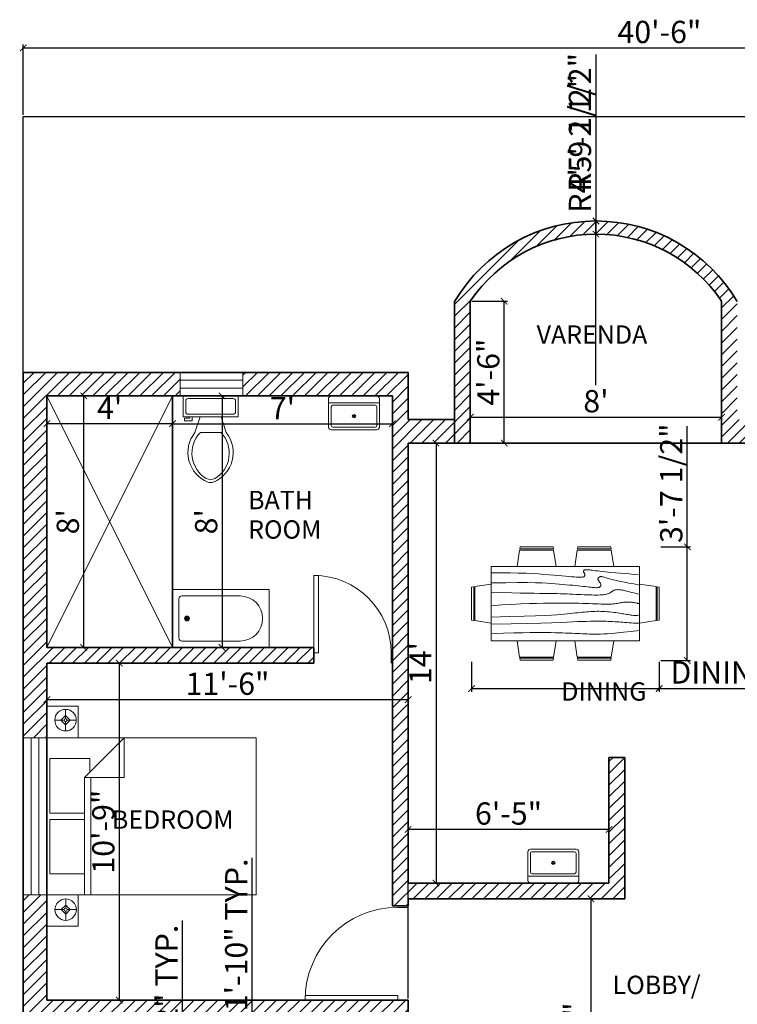
# Model space of a CAD drawing. Units: inches. Extents: x 3799 to 20199, y 1682 to 8087.
# Tile 19 of 30: x 14308 to 14582, y 2852 to 3227. Entities that reach past the tile are written whole.
import ezdxf

# ---------------------------------------------------------------- set-up
doc = ezdxf.new("R2010")
doc.units = ezdxf.units.IN
for name, color, linetype, lineweight in [('A-ANNO-DIMS', 2, 'Continuous', 18), ('A-AREA-IDEN', 7, 'Continuous', 18), ('A-DOOR', 3, 'Continuous', 18), ('A-FLOR-FIXT', 9, 'Continuous', 18), ('A-FURN', 8, 'Continuous', 18), ('A-GLAZ', 152, 'Continuous', 18), ('A-WALL', 7, 'Continuous', 35), ('A-WALL-PATT', 252, 'Continuous', 13), ('C-PROP', 7, 'Continuous', 25)]:
    doc.layers.add(name, color=color, linetype=linetype, lineweight=lineweight)
doc.styles.get("Standard").update_dxf_attribs({"font": 'arial.ttf'})
doc.dimstyles.new('ISO-25', dxfattribs={"dimtxt": 8.5, "dimasz": 2.5, "dimexe": 1.25, "dimexo": 0.625, "dimtad": 1, "dimdec": 0, "dimlunit": 3, "dimtxsty": 'Standard', "dimblk": 'ARCHTICK', "dimcen": 2.5, "dimadec": 0, "dimazin": 0, "dimtfac": 1, "dimtdec": 0, "dimtmove": 0, "dimatfit": 3, "dimfxl": 1, "dimarcsym": 0})

# ---------------------------------------------------------------- blocks, each defined once
blk = doc.blocks.new('Bed - Queen')
for p, q in [((0, -80.00003), (0, 0)), ((0, 0), (59.99999, 0)), ((59.99999, 0), (59.99999, -80.00003)), ((7.99999, -1.2), (28.79998, -1.2)), ((7.99999, -14.4), (7.99999, -1.2)), ((28.79998, -1.2), (28.79998, -14.4)), ((31.19999, -1.2), (51.99999, -1.2)), ((31.19999, -14.4), (31.19999, -1.2)), ((51.99999, -1.2), (51.99999, -16.4)), ((0, -14.4), (44.8, -14.4)), ((59.99999, -29.6), (44.8, -14.4)), ((44.8, -14.4), (44.8, -29.6)), ((44.8, -16.8), (0, -16.8)), ((51.99999, -16.4), (46.79936, -16.4)), ((44.8, -29.6), (59.99999, -29.6)), ((59.99999, -80.00003), (0, -80.00003))]:
    blk.add_line(p, q)
blk = doc.blocks.new('*U7')
for p, q in [((0, 0), (0, -100)), ((750, 0), (750, -100))]:
    blk.add_line(p, q)
blk.add_lwpolyline([(0, 0), (0, 750), (43.75, 750), (43.75, 0)], close=True)
blk.add_arc((0, 0), 750, 0, 90)
blk = doc.blocks.new('*U16')
for p, q in [((0, 0), (0, -100)), ((900, 0), (900, -100))]:
    blk.add_line(p, q)
blk.add_lwpolyline([(0, 0), (0, 900), (43.75, 900), (43.75, 0)], close=True)
blk.add_arc((0, 0), 900, 0, 90)
blk = doc.blocks.new('Bath Tub - 26 x 60 in.')
for p, q in [((8, -18), (10, -18)), ((9, -17), (9, -19))]:
    blk.add_line(p, q)
blk.add_lwpolyline([(0, -36), (0, 0), (60, 0), (60, -36)], close=True)
for points in [[(4, -30), (4, -6)], [(6, -4), (42, -4)], [(42, -32), (6, -32)]]:
    blk.add_lwpolyline(points)
for radius in [1.5, 1]:
    blk.add_circle((9, -18), radius)
for centre, radius, start, end in [((5.75, -5.75), 1.77, 81.8699, 188.1301), ((42, -18), 14, 270, 90), ((5.75, -30.25), 1.77, 171.8699, 278.1301)]:
    blk.add_arc(centre, radius, start, end)
blk = doc.blocks.new('Sink-single - 30 in top')
blk.add_line((-15, -3.999996), (15, -3.999996))
for points in [[(-13.5, 0), (13.5, 0)], [(-15, -18.499996), (-15, -1.5)], [(-12.5, -5.499996), (12.5, -5.499996)], [(15, -1.5), (15, -18.499996)], [(-13.5, -17.499996), (-13.5, -6.499996)], [(13.5, -6.499996), (13.5, -17.499996)], [(13.5, -19.999996), (-13.5, -19.999996)], [(12.5, -18.499996), (-12.5, -18.499996)]]:
    blk.add_lwpolyline(points)
for radius in [1, 0.5]:
    blk.add_circle((0, -11.999996), radius)
for centre, radius, start, end in [((-13.5, -1.5), 1.5, 90, 180), ((-12.5, -6.499996), 1, 90, 180), ((12.5, -6.499996), 1, 0, 90), ((13.5, -1.5), 1.5, 0, 90), ((-13.5, -18.499996), 1.5, 180, 270), ((-12.5, -17.499996), 1, 180, 270), ((12.5, -17.499996), 1, 270, 0), ((13.5, -18.499996), 1.5, 270, 0)]:
    blk.add_arc(centre, radius, start, end)
blk = doc.blocks.new('Dining Set - 36 x 72 in.')
for p, q in [((-22.2343, 26.00059), (-23.4847, 17.99762)), ((-22.2304, 26), (-5.7608, 26)), ((-22, 27.5), (-22.1562, 26.50042)), ((-5.8416, 26.5), (-22.1534, 26.5)), ((-22, 27.5), (-6, 27.5)), ((-5.8437, 26.49966), (-6, 27.5)), ((-4.5152, 17.99762), (-5.7655, 25.99926)), ((5.7657, 26.00059), (4.5153, 17.99762)), ((5.7696, 26), (22.2392, 26)), ((6, 27.5), (5.8438, 26.50042)), ((22.1584, 26.5), (5.8466, 26.5)), ((6, 27.5), (22, 27.5)), ((22.1563, 26.49966), (22, 27.5)), ((23.4848, 17.99762), (22.2345, 25.99926)), ((36, 18), (-36, 18)), ((-36, 18), (-36, -18)), ((36, -18), (36, 18)), ((-45.5, 8), (-44.5004, 8.15617)), ((-45.5, 8), (-45.5, -8)), ((-44.5, -8.15843), (-44.5, 8.15338)), ((-44.0006, 8.23428), (-35.9976, 9.48474)), ((-44, 8.23041), (-44, -8.23915)), ((44.0006, 8.23428), (35.9976, 9.48474)), ((44, 8.23041), (44, -8.23915)), ((44.5, -8.15843), (44.5, 8.15338)), ((45.5, 8), (44.5005, 8.15617)), ((45.5, 8), (45.5, -8)), ((-44.4997, -8.15631), (-45.5, -8)), ((-35.9976, -9.48476), (-43.9993, -8.2345)), ((35.9976, -9.48476), (43.9993, -8.2345)), ((44.4997, -8.15631), (45.5, -8)), ((-36, -18), (36, -18)), ((-22.2343, -26.0006), (-23.4847, -17.99762)), ((-4.5152, -17.99762), (-5.7655, -25.99928)), ((5.7657, -26.0006), (4.5153, -17.99762)), ((23.4848, -17.99762), (22.2345, -25.99928)), ((-22.2304, -26), (-5.7608, -26)), ((-22, -27.5), (-22.1562, -26.50044)), ((-5.8416, -26.5), (-22.1534, -26.5)), ((-22, -27.5), (-6, -27.5)), ((-5.8437, -26.49967), (-6, -27.5)), ((5.7696, -26), (22.2392, -26)), ((6, -27.5), (5.8438, -26.50044)), ((22.1584, -26.5), (5.8466, -26.5)), ((6, -27.5), (22, -27.5)), ((22.1563, -26.49967), (22, -27.5))]:
    blk.add_line(p, q)
for points in [[(-36, 15), (-31.1772, 14.97754), (-26.8079, 14.91406), (-22.8538, 14.81543), (-19.276, 14.6875), (-16.0362, 14.53613), (-13.0957, 14.36718), (-10.4159, 14.18652), (-7.9583, 14), (-5.6904, 13.81315), (-3.6035, 13.63021), (-1.6954, 13.45508), (0.0365, 13.29166), (1.5945, 13.14388), (2.9811, 13.01562), (4.1988, 12.9108), (5.25, 12.83333), (6.1393, 12.78613), (6.8802, 12.76823), (7.4883, 12.77767), (7.9792, 12.8125), (8.3685, 12.87077), (8.6719, 12.95052), (8.9049, 13.0498), (9.0833, 13.16666), (9.2205, 13.29899), (9.3216, 13.44401), (9.3895, 13.59879), (9.4271, 13.76041), (9.4373, 13.92594), (9.4232, 14.09245), (9.3875, 14.257), (9.3333, 14.41666), (9.2638, 14.56917), (9.1836, 14.71484), (9.0975, 14.85465), (9.0104, 14.98958), (8.9272, 15.1206), (8.8529, 15.2487), (8.7922, 15.37483), (8.75, 15.5), (8.7305, 15.62467), (8.7344, 15.74739), (8.7617, 15.86621), (8.8125, 15.97916), (8.8867, 16.08431), (8.9844, 16.17968), (9.1055, 16.26334), (9.25, 16.33333), (9.4189, 16.38802), (9.6172, 16.42708), (9.8506, 16.45052), (10.125, 16.45833), (10.4463, 16.45052), (10.8203, 16.42708), (11.2529, 16.38802), (11.75, 16.33333), (12.3184, 16.26318), (12.9694, 16.17838), (13.7151, 16.07991), (14.5677, 15.96875), (15.5395, 15.84586), (16.6426, 15.71224), (17.8893, 15.56884), (19.2917, 15.41666), (20.859, 15.25667), (22.5879, 15.08984), (24.4721, 14.91715), (26.5052, 14.73958), (28.6809, 14.5581), (30.9929, 14.3737), (33.4347, 14.18733), (36, 14)], [(-36, 10), (-28.9766, 10.14274), (-23.1725, 10.20442), (-18.4241, 10.19775), (-14.5677, 10.13541), (-11.4399, 10.03011), (-8.877, 9.89453), (-6.7154, 9.74137), (-4.7917, 9.58333), (-2.9698, 9.43082), (-1.2246, 9.28515), (0.4415, 9.14534), (2.026, 9.01041), (3.5266, 8.87939), (4.9408, 8.7513), (6.266, 8.62516), (7.5, 8.5), (8.6411, 8.37549), (9.6914, 8.2539), (10.6538, 8.13818), (11.5312, 8.03125), (12.3267, 7.93603), (13.043, 7.85547), (13.6831, 7.79248), (14.25, 7.75), (14.7471, 7.7303), (15.1797, 7.73307), (15.5537, 7.75732), (15.875, 7.80208), (16.1494, 7.86637), (16.3828, 7.94922), (16.5811, 8.04964), (16.75, 8.16666), (16.8944, 8.29915), (17.0143, 8.44531), (17.1089, 8.60319), (17.1771, 8.77083), (17.218, 8.94629), (17.2305, 9.1276), (17.2137, 9.31282), (17.1667, 9.5), (17.0895, 9.6875), (16.987, 9.875), (16.8649, 10.0625), (16.7292, 10.25), (16.5856, 10.4375), (16.4401, 10.625), (16.2985, 10.8125), (16.1667, 11), (16.05, 11.18733), (15.9518, 11.3737), (15.8752, 11.5581), (15.8229, 11.73958), (15.798, 11.91715), (15.8034, 12.08984), (15.842, 12.25667), (15.9167, 12.41666), (16.0295, 12.56836), (16.1784, 12.70833), (16.3605, 12.83268), (16.5729, 12.9375), (16.8127, 13.01888), (17.0768, 13.07291), (17.3625, 13.0957), (17.6667, 13.08333), (17.9894, 13.03312), (18.3418, 12.94726), (18.7382, 12.82918), (19.1927, 12.68229), (19.7195, 12.51001), (20.3327, 12.31575), (21.0465, 12.10294), (21.875, 11.875), (22.8357, 11.63354), (23.959, 11.37304), (25.2786, 11.08618), (26.8282, 10.76562), (28.6414, 10.40405), (30.752, 9.99414), (33.1936, 9.52856), (36, 9)], [(-36, 5.5), (-30.7157, 5.3348), (-26.069, 5.20963), (-21.9946, 5.11767), (-18.4271, 5.05208), (-15.3009, 5.00602), (-12.5508, 4.97265), (-10.1112, 4.94515), (-7.9167, 4.91666), (-5.909, 4.88167), (-4.0586, 4.83984), (-2.3429, 4.79215), (-0.7396, 4.73958), (0.7739, 4.6831), (2.22, 4.6237), (3.6213, 4.56233), (5, 4.5), (6.373, 4.43782), (7.7344, 4.3776), (9.0723, 4.32129), (10.375, 4.27083), (11.6309, 4.22819), (12.8281, 4.19531), (13.9551, 4.17415), (15, 4.16666), (15.954, 4.17448), (16.819, 4.19791), (17.6001, 4.23698), (18.3021, 4.29166), (18.9299, 4.36198), (19.4883, 4.44791), (19.9823, 4.54948), (20.4167, 4.66666), (20.7969, 4.79899), (21.1302, 4.94401), (21.4245, 5.09879), (21.6875, 5.26041), (21.9271, 5.42594), (22.1511, 5.59245), (22.3672, 5.757), (22.5834, 5.91666), (22.8065, 6.06868), (23.0404, 6.21093), (23.2879, 6.34147), (23.5521, 6.45833), (23.8358, 6.55957), (24.142, 6.64323), (24.4735, 6.70735), (24.8334, 6.75), (25.2235, 6.76969), (25.642, 6.76692), (26.0858, 6.74267), (26.5521, 6.69791), (27.0379, 6.63362), (27.5404, 6.55078), (28.0565, 6.45036), (28.5834, 6.33333), (29.1242, 6.19987), (29.7071, 6.04687), (30.3661, 5.87044), (31.1354, 5.66666), (32.0493, 5.43164), (33.142, 5.16146), (34.4475, 4.85221), (36, 4.5)], [(-36, -1), (-30.7915, -0.6591), (-26.0195, -0.38216), (-21.6519, -0.16284), (-17.6563, 0.00521), (-14.0005, 0.12833), (-10.6523, 0.21289), (-7.5796, 0.26522), (-4.75, 0.29166), (-2.134, 0.29793), (0.2878, 0.28711), (2.5317, 0.26163), (4.6146, 0.22396), (6.5529, 0.17651), (8.3633, 0.12174), (10.0623, 0.06209), (11.6667, 0), (13.1899, -0.06201), (14.6341, -0.1211), (15.9982, -0.17432), (17.2813, -0.21875), (18.4823, -0.25147), (19.6003, -0.26953), (20.6343, -0.27002), (21.5834, -0.25), (22.4481, -0.20768), (23.2357, -0.14584), (23.9549, -0.06836), (24.6146, 0.02083), (25.2235, 0.11784), (25.7904, 0.21875), (26.3241, 0.31966), (26.8334, 0.41666), (27.3265, 0.50618), (27.8099, 0.58593), (28.2894, 0.65397), (28.7709, 0.70833), (29.2601, 0.74707), (29.763, 0.76823), (30.2855, 0.76985), (30.8334, 0.75), (31.4088, 0.70784), (31.9994, 0.64713), (32.589, 0.57275), (33.1615, 0.48958), (33.7008, 0.4025), (34.1908, 0.3164), (34.6153, 0.23616), (34.9584, 0.16666), (35.2099, 0.11165), (35.3848, 0.07031), (35.504, 0.04069), (35.5886, 0.02083), (35.6594, 0.00879), (35.7377, 0.0026), (35.8442, 0.00032), (36, 0)], [(-36, -6.5), (-27.1843, -6.31267), (-20.084, -6.1263), (-14.469, -5.9419), (-10.1094, -5.76042), (-6.7752, -5.58285), (-4.2363, -5.41016), (-2.2629, -5.24333), (-0.625, -5.08334), (0.8708, -4.93099), (2.2715, -4.78646), (3.5872, -4.64974), (4.8281, -4.52084), (6.0046, -4.39974), (7.127, -4.28646), (8.2053, -4.18099), (9.25, -4.08334), (10.2705, -3.99382), (11.2734, -3.91407), (12.2647, -3.84603), (13.25, -3.79167), (14.2354, -3.75293), (15.2266, -3.73177), (16.2295, -3.73015), (17.25, -3.75), (18.2912, -3.79248), (19.3451, -3.85547), (20.4009, -3.93604), (21.4479, -4.03125), (22.4754, -4.13819), (23.4727, -4.25391), (24.4289, -4.37549), (25.3334, -4.5), (26.1785, -4.62492), (26.9694, -4.74935), (27.7145, -4.87281), (28.4219, -4.99479), (29.1, -5.11483), (29.7572, -5.23242), (30.4016, -5.34709), (31.0417, -5.45834), (31.6837, -5.56437), (32.3262, -5.65821), (32.9658, -5.73153), (33.599, -5.77604), (34.2224, -5.78345), (34.8327, -5.74545), (35.4264, -5.65373), (36, -5.5)], [(-36, -10), (-26.4022, -9.81299), (-18.4675, -9.62891), (-11.9839, -9.45069), (-6.7396, -9.28125), (-2.5226, -9.12354), (0.8789, -8.98047), (3.6769, -8.85498), (6.0833, -8.75), (8.2767, -8.66765), (10.3021, -8.60677), (12.1712, -8.56543), (13.8958, -8.54167), (15.4876, -8.53353), (16.9583, -8.53907), (18.3197, -8.55632), (19.5834, -8.58334), (20.7616, -8.61841), (21.8685, -8.66081), (22.9188, -8.71004), (23.9271, -8.76563), (24.9081, -8.82707), (25.8763, -8.89388), (26.8465, -8.96558), (27.8334, -9.04167), (28.8474, -9.12118), (29.8828, -9.20117), (30.93, -9.27824), (31.9792, -9.34896), (33.0205, -9.40991), (34.0443, -9.45768), (35.0407, -9.48885), (36, -9.5)], [(-36, -14.5), (-30.0881, -14.33513), (-25.0332, -14.21224), (-20.7312, -14.12647), (-17.0781, -14.07292), (-13.97, -14.04671), (-11.3027, -14.04297), (-8.9724, -14.05681), (-6.875, -14.08334), (-4.9224, -14.11833), (-3.0905, -14.16016), (-1.3709, -14.20785), (0.2448, -14.26042), (1.7647, -14.3169), (3.1973, -14.3763), (4.5507, -14.43767), (5.8333, -14.5), (7.0554, -14.5621), (8.235, -14.62175), (9.3922, -14.67652), (10.5469, -14.72396), (11.7192, -14.76164), (12.929, -14.78711), (14.1965, -14.79794), (15.5417, -14.79167), (16.9933, -14.76424), (18.6152, -14.70508), (20.4804, -14.60197), (22.6615, -14.44271), (25.2312, -14.21509), (28.2624, -13.9069), (31.8277, -13.50594), (36, -13)]]:
    blk.add_lwpolyline(points)
blk = doc.blocks.new('Toilet - top')
for p, q in [((9.5, -6), (9.5, -2)), ((-10, -8.5), (-8, -8.5)), ((-10, -9.5), (-10, -8.5)), ((-7, -9.5), (-10, -9.5)), ((-8, -8.5), (-8, -8)), ((-7, -8), (-7, -9.5)), ((-4, -8), (-6, -14)), ((4, -8), (6, -14)), ((4, -14), (-4, -14))]:
    blk.add_line(p, q)
blk.add_lwpolyline([(10.5, -8), (10.5, 0), (-10.5, 0), (-10.5, -8)], close=True)
for points in [[(-9.5, -2), (-9.5, -6)], [(8.5, -1), (-8.5, -1)], [(-8.5, -7), (8.5, -7)]]:
    blk.add_lwpolyline(points)
for centre, radius, start, end in [((-8.62, -1.88), 0.884, 81.8699, 188.1301), ((8.62, -1.88), 0.884, 351.8699, 98.1301), ((-8.62, -6.12), 0.884, 171.8699, 278.1301), ((8.62, -6.12), 0.884, 261.8699, 8.1301), ((3.52, -21.58), 12.17, 141.4691, 247.9714), ((4.2, -21.82), 11.33, 136.3677, 238.9468), ((-3.52, -21.58), 12.17, 292.0284, 38.5307), ((-4.2, -21.82), 11.33, 301.053, 43.6321), ((0, -27.88), 4, 245.7318, 294.2682), ((0, -29), 4, 254.8605, 285.1395)]:
    blk.add_arc(centre, radius, start, end)
blk = doc.blocks.new('Lamp - Table')
for p, q in [((0, 7), (0, 1)), ((-1, 0), (-7, 0)), ((0, 3), (-3, 0)), ((-3, 0), (0, -3)), ((3, 0), (0, 3)), ((0, -3), (3, 0)), ((1, 0), (7, 0)), ((0, -1), (0, -7))]:
    blk.add_line(p, q)
for radius in [7, 1]:
    blk.add_circle((0, 0), radius)
blk = doc.blocks.new('_ArchTick')
at = {"color": 0, "linetype": 'ByBlock', "const_width": 0.15}
blk.add_lwpolyline([(-0.5, -0.5), (0.5, 0.5)], dxfattribs=at)
blk = doc.blocks.new('*D99')
at = {"layer": 'A-ANNO-DIMS', "color": 0, "lineweight": -2, "transparency": 16777216}
for p, q in [((14318.46, 3083.13), (14318.46, 3071.99)), ((14366.46, 3083.13), (14366.46, 3071.99)), ((14318.46, 3073.24), (14366.46, 3073.24))]:
    blk.add_line(p, q, dxfattribs=at)
at = {"layer": 'Defpoints', "color": 0, "transparency": 16777216}
for p in [(14318.46, 3083.76), (14366.46, 3083.76), (14366.46, 3073.24)]:
    blk.add_point(p, dxfattribs=at)
at = {"layer": 'A-ANNO-DIMS', "color": 0, "lineweight": -2, "transparency": 16777216, "xscale": 2.5, "yscale": 2.5, "zscale": 2.5, "rotation": 180}
blk.add_blockref('_ArchTick', (14318.46, 3073.24), dxfattribs=at)
at = {"layer": 'A-ANNO-DIMS', "color": 0, "lineweight": -2, "transparency": 16777216, "xscale": 2.5, "yscale": 2.5, "zscale": 2.5}
blk.add_blockref('_ArchTick', (14366.46, 3073.24), dxfattribs=at)
at = {"layer": 'A-ANNO-DIMS', "color": 0, "transparency": 16777216, "insert": (14342.46, 3078.12), "char_height": 8.5, "attachment_point": 5}
blk.add_mtext("4'", dxfattribs=at)
blk = doc.blocks.new('*D100')
at = {"layer": 'A-ANNO-DIMS', "color": 0, "lineweight": -2, "transparency": 16777216}
for p, q in [((14319.09, 3083.76), (14333.79, 3083.76)), ((14332.54, 2987.76), (14332.54, 3083.76)), ((14319.09, 2987.76), (14333.79, 2987.76))]:
    blk.add_line(p, q, dxfattribs=at)
at = {"layer": 'Defpoints', "color": 0, "transparency": 16777216}
for p in [(14318.46, 3083.76), (14332.54, 3083.76), (14318.46, 2987.76)]:
    blk.add_point(p, dxfattribs=at)
at = {"layer": 'A-ANNO-DIMS', "color": 0, "lineweight": -2, "transparency": 16777216, "xscale": 2.5, "yscale": 2.5, "zscale": 2.5}
for p, rotation in [((14332.54, 3083.76), 90), ((14332.54, 2987.76), 270)]:
    blk.add_blockref('_ArchTick', p, dxfattribs=dict(at, rotation=rotation))
at = {"layer": 'A-ANNO-DIMS', "color": 0, "transparency": 16777216, "insert": (14327.58, 3035.76), "char_height": 8.5, "attachment_point": 5, "rotation": 90}
blk.add_mtext("8'", dxfattribs=at)
blk = doc.blocks.new('*D101')
at = {"layer": 'A-ANNO-DIMS', "color": 0, "lineweight": -2, "transparency": 16777216}
for p, q in [((14366.46, 3083.13), (14366.46, 3071.9)), ((14450.46, 3083.13), (14450.46, 3071.9)), ((14366.46, 3073.15), (14450.46, 3073.15))]:
    blk.add_line(p, q, dxfattribs=at)
at = {"layer": 'Defpoints', "color": 0, "transparency": 16777216}
for p in [(14366.46, 3083.76), (14450.46, 3083.76), (14450.46, 3073.15)]:
    blk.add_point(p, dxfattribs=at)
at = {"layer": 'A-ANNO-DIMS', "color": 0, "lineweight": -2, "transparency": 16777216, "xscale": 2.5, "yscale": 2.5, "zscale": 2.5, "rotation": 180}
blk.add_blockref('_ArchTick', (14366.46, 3073.15), dxfattribs=at)
at = {"layer": 'A-ANNO-DIMS', "color": 0, "lineweight": -2, "transparency": 16777216, "xscale": 2.5, "yscale": 2.5, "zscale": 2.5}
blk.add_blockref('_ArchTick', (14450.46, 3073.15), dxfattribs=at)
at = {"layer": 'A-ANNO-DIMS', "color": 0, "transparency": 16777216, "insert": (14408.46, 3078.03), "char_height": 8.5, "attachment_point": 5}
blk.add_mtext("7'", dxfattribs=at)
blk = doc.blocks.new('*D102')
at = {"layer": 'A-ANNO-DIMS', "color": 0, "lineweight": -2, "transparency": 16777216}
for p, q in [((14367.09, 3083.76), (14386.64, 3083.76)), ((14385.39, 3083.76), (14385.39, 2987.76)), ((14367.09, 2987.76), (14386.64, 2987.76))]:
    blk.add_line(p, q, dxfattribs=at)
at = {"layer": 'Defpoints', "color": 0, "transparency": 16777216}
for p in [(14366.46, 3083.76), (14366.46, 2987.76), (14385.39, 2987.76)]:
    blk.add_point(p, dxfattribs=at)
at = {"layer": 'A-ANNO-DIMS', "color": 0, "lineweight": -2, "transparency": 16777216, "xscale": 2.5, "yscale": 2.5, "zscale": 2.5}
for p, rotation in [((14385.39, 3083.76), 90), ((14385.39, 2987.76), 270)]:
    blk.add_blockref('_ArchTick', p, dxfattribs=dict(at, rotation=rotation))
at = {"layer": 'A-ANNO-DIMS', "color": 0, "transparency": 16777216, "insert": (14380.42, 3035.76), "char_height": 8.5, "attachment_point": 5, "rotation": 90}
blk.add_mtext("8'", dxfattribs=at)
blk = doc.blocks.new('*D103')
at = {"layer": 'A-ANNO-DIMS', "color": 0, "lineweight": -2, "transparency": 16777216}
for p, q in [((14318.46, 2853.72), (14318.46, 2969.09)), ((14318.46, 2967.84), (14456.46, 2967.84)), ((14456.46, 2853.72), (14456.46, 2969.09))]:
    blk.add_line(p, q, dxfattribs=at)
at = {"layer": 'Defpoints', "color": 0, "transparency": 16777216}
for p in [(14456.46, 2967.84), (14318.46, 2853.09), (14456.46, 2853.09)]:
    blk.add_point(p, dxfattribs=at)
at = {"layer": 'A-ANNO-DIMS', "color": 0, "lineweight": -2, "transparency": 16777216, "xscale": 2.5, "yscale": 2.5, "zscale": 2.5, "rotation": 180}
blk.add_blockref('_ArchTick', (14318.46, 2967.84), dxfattribs=at)
at = {"layer": 'A-ANNO-DIMS', "color": 0, "lineweight": -2, "transparency": 16777216, "xscale": 2.5, "yscale": 2.5, "zscale": 2.5}
blk.add_blockref('_ArchTick', (14456.46, 2967.84), dxfattribs=at)
at = {"layer": 'A-ANNO-DIMS', "color": 0, "transparency": 16777216, "insert": (14387.46, 2972.81), "char_height": 8.5, "attachment_point": 5}
blk.add_mtext('11\'-6"', dxfattribs=at)
blk = doc.blocks.new('*D104')
at = {"layer": 'A-ANNO-DIMS', "color": 0, "lineweight": -2, "transparency": 16777216}
for p, q in [((14319.09, 2981.76), (14347.35, 2981.76)), ((14346.1, 2981.76), (14346.1, 2853.09)), ((14319.09, 2853.09), (14347.35, 2853.09))]:
    blk.add_line(p, q, dxfattribs=at)
at = {"layer": 'Defpoints', "color": 0, "transparency": 16777216}
for p in [(14318.46, 2981.76), (14318.46, 2853.09), (14346.1, 2853.09)]:
    blk.add_point(p, dxfattribs=at)
at = {"layer": 'A-ANNO-DIMS', "color": 0, "lineweight": -2, "transparency": 16777216, "xscale": 2.5, "yscale": 2.5, "zscale": 2.5}
for p, rotation in [((14346.1, 2981.76), 90), ((14346.1, 2853.09), 270)]:
    blk.add_blockref('_ArchTick', p, dxfattribs=dict(at, rotation=rotation))
at = {"layer": 'A-ANNO-DIMS', "color": 0, "transparency": 16777216, "insert": (14341.14, 2917.42), "char_height": 8.5, "attachment_point": 5, "rotation": 90}
blk.add_mtext('10\'-9"', dxfattribs=at)
blk = doc.blocks.new('*D112')
at = {"layer": 'A-ANNO-DIMS', "color": 0, "lineweight": -2, "transparency": 16777216}
for p, q in [((14538.58, 2891.79), (14525.03, 2891.79)), ((14526.28, 2891.79), (14526.28, 2787.09)), ((14538.58, 2787.09), (14525.03, 2787.09))]:
    blk.add_line(p, q, dxfattribs=at)
at = {"layer": 'Defpoints', "color": 0, "transparency": 16777216}
for p in [(14539.2, 2891.79), (14526.28, 2787.09), (14539.2, 2787.09)]:
    blk.add_point(p, dxfattribs=at)
at = {"layer": 'A-ANNO-DIMS', "color": 0, "lineweight": -2, "transparency": 16777216, "xscale": 2.5, "yscale": 2.5, "zscale": 2.5}
for p, rotation in [((14526.28, 2891.79), 90), ((14526.28, 2787.09), 270)]:
    blk.add_blockref('_ArchTick', p, dxfattribs=dict(at, rotation=rotation))
at = {"layer": 'A-ANNO-DIMS', "color": 0, "transparency": 16777216, "insert": (14521.32, 2839.44), "char_height": 8.5, "attachment_point": 5, "rotation": 90}
blk.add_mtext('8\'-9"', dxfattribs=at)
blk = doc.blocks.new('*D113')
at = {"layer": 'A-ANNO-DIMS', "color": 0, "lineweight": -2, "transparency": 16777216}
for p, q in [((14456.46, 2945.16), (14456.46, 2917.03)), ((14533.2, 2945.16), (14533.2, 2917.03)), ((14533.2, 2918.28), (14456.46, 2918.28))]:
    blk.add_line(p, q, dxfattribs=at)
at = {"layer": 'Defpoints', "color": 0, "transparency": 16777216}
for p in [(14456.46, 2945.79), (14533.2, 2945.79), (14456.46, 2918.28)]:
    blk.add_point(p, dxfattribs=at)
at = {"layer": 'A-ANNO-DIMS', "color": 0, "lineweight": -2, "transparency": 16777216, "xscale": 2.5, "yscale": 2.5, "zscale": 2.5, "rotation": 180}
blk.add_blockref('_ArchTick', (14456.46, 2918.28), dxfattribs=at)
at = {"layer": 'A-ANNO-DIMS', "color": 0, "lineweight": -2, "transparency": 16777216, "xscale": 2.5, "yscale": 2.5, "zscale": 2.5}
blk.add_blockref('_ArchTick', (14533.2, 2918.28), dxfattribs=at)
at = {"layer": 'A-ANNO-DIMS', "color": 0, "transparency": 16777216, "insert": (14494.83, 2923.25), "char_height": 8.5, "attachment_point": 5}
blk.add_mtext('6\'-5"', dxfattribs=at)
blk = doc.blocks.new('*D114')
at = {"layer": 'A-ANNO-DIMS', "color": 0, "lineweight": -2, "transparency": 16777216}
for p, q in [((14457.09, 3065.79), (14468.38, 3065.79)), ((14467.13, 3065.79), (14467.13, 2897.79)), ((14457.09, 2897.79), (14468.38, 2897.79))]:
    blk.add_line(p, q, dxfattribs=at)
at = {"layer": 'Defpoints', "color": 0, "transparency": 16777216}
for p in [(14456.46, 3065.79), (14456.46, 2897.79), (14467.13, 2897.79)]:
    blk.add_point(p, dxfattribs=at)
at = {"layer": 'A-ANNO-DIMS', "color": 0, "lineweight": -2, "transparency": 16777216, "xscale": 2.5, "yscale": 2.5, "zscale": 2.5}
for p, rotation in [((14467.13, 3065.79), 90), ((14467.13, 2897.79), 270)]:
    blk.add_blockref('_ArchTick', p, dxfattribs=dict(at, rotation=rotation))
at = {"layer": 'A-ANNO-DIMS', "color": 0, "transparency": 16777216, "insert": (14462.23, 2981.79), "char_height": 8.5, "attachment_point": 5, "rotation": 90}
blk.add_mtext("14'", dxfattribs=at)
blk = doc.blocks.new('*D115')
at = {"layer": 'A-ANNO-DIMS', "color": 0, "lineweight": -2, "transparency": 16777216}
for p, q in [((14480.85, 3119.94), (14494.42, 3119.94)), ((14493.17, 3065.79), (14493.17, 3119.94)), ((14480.85, 3065.79), (14494.42, 3065.79))]:
    blk.add_line(p, q, dxfattribs=at)
at = {"layer": 'Defpoints', "color": 0, "transparency": 16777216}
for p in [(14480.23, 3119.94), (14493.17, 3119.94), (14480.23, 3065.79)]:
    blk.add_point(p, dxfattribs=at)
at = {"layer": 'A-ANNO-DIMS', "color": 0, "lineweight": -2, "transparency": 16777216, "xscale": 2.5, "yscale": 2.5, "zscale": 2.5}
for p, rotation in [((14493.17, 3119.94), 90), ((14493.17, 3065.79), 270)]:
    blk.add_blockref('_ArchTick', p, dxfattribs=dict(at, rotation=rotation))
at = {"layer": 'A-ANNO-DIMS', "color": 0, "transparency": 16777216, "insert": (14488.21, 3092.86), "char_height": 8.5, "attachment_point": 5, "rotation": 90}
blk.add_mtext('4\'-6"', dxfattribs=at)
blk = doc.blocks.new('*D116')
at = {"layer": 'A-ANNO-DIMS', "color": 0, "lineweight": -2, "transparency": 16777216}
for p, q in [((14480.23, 3066.41), (14480.23, 3076.95)), ((14480.23, 3075.7), (14576.23, 3075.7)), ((14576.23, 3066.41), (14576.23, 3076.95))]:
    blk.add_line(p, q, dxfattribs=at)
at = {"layer": 'Defpoints', "color": 0, "transparency": 16777216}
for p in [(14576.23, 3075.7), (14480.23, 3065.79), (14576.23, 3065.79)]:
    blk.add_point(p, dxfattribs=at)
at = {"layer": 'A-ANNO-DIMS', "color": 0, "lineweight": -2, "transparency": 16777216, "xscale": 2.5, "yscale": 2.5, "zscale": 2.5, "rotation": 180}
blk.add_blockref('_ArchTick', (14480.23, 3075.7), dxfattribs=at)
at = {"layer": 'A-ANNO-DIMS', "color": 0, "lineweight": -2, "transparency": 16777216, "xscale": 2.5, "yscale": 2.5, "zscale": 2.5}
blk.add_blockref('_ArchTick', (14576.23, 3075.7), dxfattribs=at)
at = {"layer": 'A-ANNO-DIMS', "color": 0, "transparency": 16777216, "insert": (14528.23, 3080.67), "char_height": 8.5, "attachment_point": 5}
blk.add_mtext("8'", dxfattribs=at)
blk = doc.blocks.new('*D122')
at = {"layer": 'A-ANNO-DIMS', "color": 0, "lineweight": -2, "transparency": 16777216}
for p, q in [((14309.46, 3191.05), (14309.46, 3217.92)), ((14795.46, 3191.05), (14795.46, 3217.92)), ((14309.46, 3216.67), (14795.46, 3216.67))]:
    blk.add_line(p, q, dxfattribs=at)
at = {"layer": 'Defpoints', "color": 0, "transparency": 16777216}
for p in [(14795.46, 3216.67), (14309.46, 3190.42), (14795.46, 3190.42)]:
    blk.add_point(p, dxfattribs=at)
at = {"layer": 'A-ANNO-DIMS', "color": 0, "lineweight": -2, "transparency": 16777216, "xscale": 2.5, "yscale": 2.5, "zscale": 2.5, "rotation": 180}
blk.add_blockref('_ArchTick', (14309.46, 3216.67), dxfattribs=at)
at = {"layer": 'A-ANNO-DIMS', "color": 0, "lineweight": -2, "transparency": 16777216, "xscale": 2.5, "yscale": 2.5, "zscale": 2.5}
blk.add_blockref('_ArchTick', (14795.46, 3216.67), dxfattribs=at)
at = {"layer": 'A-ANNO-DIMS', "color": 0, "transparency": 16777216, "insert": (14552.46, 3221.64), "char_height": 8.5, "attachment_point": 5}
blk.add_mtext('40\'-6"', dxfattribs=at)
blk = doc.blocks.new('WIN-24IN-9IN-FRAME')
for p, q in [((0, 24), (9, 24)), ((3, 0), (3, 24)), ((6, 0), (6, 24)), ((0, 0), (9, 0))]:
    blk.add_line(p, q)
blk = doc.blocks.new('WIN-60IN-9IN-FRAME')
for p, q in [((0, 9), (0, 0)), ((60, 9), (60, 0)), ((60, 6), (0, 6)), ((60, 3), (0, 3))]:
    blk.add_line(p, q)
blk = doc.blocks.new('*D292')
at = {"layer": 'A-ANNO-DIMS', "color": 0, "lineweight": -2, "transparency": 16777216}
for p, q in [((14480.74, 2982.21), (14480.74, 2970.84)), ((14552.38, 2982.21), (14552.38, 2970.84)), ((14480.74, 2972.09), (14552.38, 2972.09)), ((14552.38, 2972.09), (14675.97, 2972.09))]:
    blk.add_line(p, q, dxfattribs=at)
at = {"layer": 'Defpoints', "color": 0, "transparency": 16777216}
for p in [(14480.74, 2982.83), (14552.38, 2982.83), (14552.38, 2972.09)]:
    blk.add_point(p, dxfattribs=at)
at = {"layer": 'A-ANNO-DIMS', "color": 0, "lineweight": -2, "transparency": 16777216, "xscale": 2.5, "yscale": 2.5, "zscale": 2.5, "rotation": 180}
blk.add_blockref('_ArchTick', (14480.74, 2972.09), dxfattribs=at)
at = {"layer": 'A-ANNO-DIMS', "color": 0, "lineweight": -2, "transparency": 16777216, "xscale": 2.5, "yscale": 2.5, "zscale": 2.5}
blk.add_blockref('_ArchTick', (14552.38, 2972.09), dxfattribs=at)
at = {"layer": 'A-ANNO-DIMS', "color": 0, "transparency": 16777216, "insert": (14615.42, 2977.11), "char_height": 8.5, "attachment_point": 5}
blk.add_mtext('DINING SET 5\'-11 1/2"', dxfattribs=at)
blk = doc.blocks.new('*D293')
at = {"layer": 'A-ANNO-DIMS', "color": 0, "lineweight": -2, "transparency": 16777216}
for p, q in [((14563.13, 3026.14), (14563.13, 3072.28)), ((14553.01, 3026.14), (14564.38, 3026.14)), ((14563.13, 2982.83), (14563.13, 3026.14)), ((14553.01, 2982.83), (14564.38, 2982.83))]:
    blk.add_line(p, q, dxfattribs=at)
at = {"layer": 'Defpoints', "color": 0, "transparency": 16777216}
for p in [(14552.38, 3026.14), (14563.13, 3026.14), (14552.38, 2982.83)]:
    blk.add_point(p, dxfattribs=at)
at = {"layer": 'A-ANNO-DIMS', "color": 0, "lineweight": -2, "transparency": 16777216, "xscale": 2.5, "yscale": 2.5, "zscale": 2.5}
for p, rotation in [((14563.13, 3026.14), 90), ((14563.13, 2982.83), 270)]:
    blk.add_blockref('_ArchTick', p, dxfattribs=dict(at, rotation=rotation))
at = {"layer": 'A-ANNO-DIMS', "color": 0, "transparency": 16777216, "insert": (14558.1, 3050.46), "char_height": 8.5, "attachment_point": 5, "rotation": 90}
blk.add_mtext('3\'-7 1/2"', dxfattribs=at)
blk = doc.blocks.new('*D305')
at = {"layer": 'A-ANNO-DIMS', "color": 0, "lineweight": -2, "transparency": 16777216}
for p, q in [((14396.87, 2846.08), (14396.87, 2907.44)), ((14391.97, 2846.08), (14398.12, 2846.08)), ((14396.87, 2823.95), (14396.87, 2846.08)), ((14391.97, 2823.95), (14398.12, 2823.95))]:
    blk.add_line(p, q, dxfattribs=at)
at = {"layer": 'Defpoints', "color": 0, "transparency": 16777216}
for p in [(14391.34, 2846.08), (14396.87, 2846.08), (14391.34, 2823.95)]:
    blk.add_point(p, dxfattribs=at)
at = {"layer": 'A-ANNO-DIMS', "color": 0, "lineweight": -2, "transparency": 16777216, "xscale": 2.5, "yscale": 2.5, "zscale": 2.5}
for p, rotation in [((14396.87, 2846.08), 90), ((14396.87, 2823.95), 270)]:
    blk.add_blockref('_ArchTick', p, dxfattribs=dict(at, rotation=rotation))
at = {"layer": 'A-ANNO-DIMS', "color": 0, "transparency": 16777216, "insert": (14391.91, 2878.01), "char_height": 8.5, "attachment_point": 5, "rotation": 90}
blk.add_mtext('1\'-10" TYP.', dxfattribs=at)
blk = doc.blocks.new('*D320')
at = {"layer": 'A-ANNO-DIMS', "color": 0, "lineweight": -2, "transparency": 16777216}
for p, q in [((14370.29, 2777.14), (14370.29, 2883.48)), ((14368.01, 2777.14), (14371.54, 2777.14)), ((14370.29, 2757.76), (14370.29, 2777.14)), ((14368.01, 2757.76), (14371.54, 2757.76))]:
    blk.add_line(p, q, dxfattribs=at)
at = {"layer": 'Defpoints', "color": 0, "transparency": 16777216}
for p in [(14367.39, 2777.14), (14370.29, 2777.14), (14367.39, 2757.76)]:
    blk.add_point(p, dxfattribs=at)
at = {"layer": 'A-ANNO-DIMS', "color": 0, "lineweight": -2, "transparency": 16777216, "xscale": 2.5, "yscale": 2.5, "zscale": 2.5}
for p, rotation in [((14370.29, 2777.14), 90), ((14370.29, 2757.76), 270)]:
    blk.add_blockref('_ArchTick', p, dxfattribs=dict(at, rotation=rotation))
at = {"layer": 'A-ANNO-DIMS', "color": 0, "transparency": 16777216, "insert": (14365.27, 2831.56), "char_height": 8.5, "attachment_point": 5, "rotation": 90}
blk.add_mtext('SINK 1\'-7 1/2" TYP.', dxfattribs=at)
blk = doc.blocks.new('*D386')
at = {"layer": 'A-ANNO-DIMS', "color": 0, "lineweight": -2, "transparency": 16777216}
for p in [(14528.23, 3214.12), (14528.23, 3087.84)]:
    blk.add_line(p, (14528.23, 3150.59), dxfattribs=at)
at = {"layer": 'Defpoints', "color": 0, "transparency": 16777216}
for p in [(14528.23, 3150.59), (14528.23, 3087.84)]:
    blk.add_point(p, dxfattribs=at)
at = {"layer": 'A-ANNO-DIMS', "color": 0, "lineweight": -2, "transparency": 16777216, "xscale": 2.5, "yscale": 2.5, "zscale": 2.5, "rotation": 269.9995589223355}
blk.add_blockref('_ArchTick', (14528.23, 3150.59), dxfattribs=at)
at = {"layer": 'A-ANNO-DIMS', "color": 0, "transparency": 16777216, "insert": (14523.21, 3188.23), "char_height": 8.5, "attachment_point": 5, "rotation": 89.9996}
blk.add_mtext('R5\'-2 1/2"', dxfattribs=at)
blk = doc.blocks.new('*D387')
at = {"layer": 'A-ANNO-DIMS', "color": 0, "lineweight": -2, "transparency": 16777216}
for p in [(14528.23, 3206.12), (14528.23, 3087.84)]:
    blk.add_line(p, (14528.23, 3145.59), dxfattribs=at)
at = {"layer": 'Defpoints', "color": 0, "transparency": 16777216}
for p in [(14528.23, 3145.59), (14528.23, 3087.84)]:
    blk.add_point(p, dxfattribs=at)
at = {"layer": 'A-ANNO-DIMS', "color": 0, "lineweight": -2, "transparency": 16777216, "xscale": 2.5, "yscale": 2.5, "zscale": 2.5, "rotation": 269.9995207281523}
blk.add_blockref('_ArchTick', (14528.23, 3145.59), dxfattribs=at)
at = {"layer": 'A-ANNO-DIMS', "color": 0, "transparency": 16777216, "insert": (14523.21, 3180.23), "char_height": 8.5, "attachment_point": 5, "rotation": 89.9995}
blk.add_mtext('R4\'-9 1/2"', dxfattribs=at)

msp = doc.modelspace()

# ---------------------------------------------------------------- hatches: boundary and pattern name
at = {"layer": 'A-WALL-PATT'}
h = msp.add_hatch(dxfattribs=at)
h.set_pattern_fill('ANSI31', color=256)
h.paths.add_polyline_path([(14318.46, 2965.3), (14318.46, 2981.76), (14420.46, 2981.76), (14420.46, 2987.76), (14318.46, 2987.76), (14318.46, 3083.76), (14369.36, 3083.76), (14369.36, 3092.76), (14309.46, 3092.76), (14309.46, 2953.3), (14318.46, 2953.3)])
h.paths.add_polyline_path([(14456.46, 3092.76), (14393.36, 3092.76), (14393.36, 3083.76), (14450.46, 3083.76), (14450.46, 2987.76), (14450.46, 2981.76), (14450.46, 2889.09), (14456.46, 2889.09), (14456.46, 2891.79), (14539.2, 2891.79), (14539.2, 2945.79), (14533.2, 2945.79), (14533.2, 2897.79), (14456.46, 2897.79), (14456.46, 3065.79), (14474.23, 3065.79), (14474.23, 3074.79), (14456.46, 3074.79)])
h.paths.add_polyline_path([(14480.23, 3119.94, -0.534305), (14576.23, 3119.94), (14576.23, 3065.79), (14582.23, 3065.79), (14582.23, 3119.79, 0.570302), (14474.23, 3119.79), (14474.23, 3065.79), (14480.23, 3065.79)])
h.paths.add_polyline_path([(14608.2, 3146.79), (14728.2, 3146.79), (14728.2, 3109.9), (14737.2, 3109.9), (14737.2, 3155.79), (14599.2, 3155.79), (14599.2, 3074.79), (14582.23, 3074.79), (14582.23, 3065.79), (14602.2, 3065.79), (14602.2, 2936.79), (14608.2, 2936.79)])
h.paths.add_polyline_path([(14737.2, 3085.9), (14728.2, 3085.9), (14728.2, 3074.79), (14638.2, 3074.79), (14638.2, 3068.79), (14728.2, 3068.79), (14728.2, 3053.38), (14737.2, 3053.38)], flags=17)
h.paths.add_polyline_path([(14737.2, 2993.38), (14728.2, 2993.38), (14728.2, 2900.79), (14599.2, 2900.79), (14599.2, 2894.79), (14737.2, 2894.79)])
h.paths.add_polyline_path([(14795.46, 2897.45), (14791.43, 2897.45), (14791.43, 2897.79), (14772.64, 2897.79), (14772.64, 2894.79), (14786.46, 2894.79), (14786.46, 2850.1), (14795.46, 2850.1)])
h.paths.add_polyline_path([(14795.46, 2826.1), (14786.46, 2826.1), (14786.46, 2787.09), (14645.38, 2787.09), (14645.38, 2781.09), (14648.46, 2781.09), (14648.46, 2740.52), (14654.46, 2740.52), (14654.46, 2781.09), (14795.46, 2781.09)])
h.paths.add_polyline_path([(14654.46, 2680.52), (14648.46, 2680.52), (14648.46, 2637.09), (14599.58, 2637.09), (14599.58, 2628.09), (14654.46, 2628.09)])
h.paths.add_polyline_path([(14539.58, 2637.09), (14504.46, 2637.09), (14504.46, 2781.09), (14609.38, 2781.09), (14609.38, 2787.09), (14498.46, 2787.09), (14498.46, 2637.09), (14456.79, 2637.09), (14456.79, 2628.09), (14539.58, 2628.09)])
h.paths.add_polyline_path([(14396.79, 2637.09), (14384.79, 2637.09), (14354.46, 2637.09), (14354.46, 2739.09), (14456.46, 2739.09), (14456.46, 2745.09), (14354.46, 2745.09), (14354.46, 2785.72), (14345.46, 2785.72), (14345.46, 2628.09), (14396.79, 2628.09)])
h.paths.add_polyline_path([(14456.46, 2853.09), (14450.46, 2853.09), (14318.46, 2853.09), (14318.46, 2893.3), (14309.46, 2893.3), (14309.46, 2847.09), (14345.46, 2847.09), (14345.46, 2809.72), (14354.46, 2809.72), (14354.46, 2847.09), (14450.46, 2847.09), (14450.46, 2775.09), (14456.46, 2775.09)])

# ---------------------------------------------------------------- linework, layer by layer
at = {"layer": 'A-FLOR-FIXT'}
for p, q in [((14318.46, 3083.76), (14366.46, 2987.76)), ((14366.46, 3083.76), (14318.46, 2987.76))]:
    msp.add_line(p, q, dxfattribs=at)
at = {"layer": 'A-FURN'}
for points in [[(14318.46, 2953.3), (14330.46, 2953.3), (14330.46, 2965.3), (14318.46, 2965.3)], [(14318.46, 2893.3), (14330.46, 2893.3), (14330.46, 2881.3), (14318.46, 2881.3)]]:
    msp.add_lwpolyline(points, close=True, dxfattribs=at)
at = {"layer": 'A-WALL'}
for p, q in [((14474.23, 3065.79), (14474.23, 3119.94)), ((14480.23, 3065.79), (14480.23, 3119.94)), ((14576.23, 3065.79), (14576.23, 3119.94)), ((14309.46, 3092.76), (14309.46, 2847.09)), ((14456.46, 3092.76), (14309.46, 3092.76)), ((14456.46, 3092.76), (14456.46, 3074.79)), ((14318.46, 3083.76), (14318.46, 2987.76)), ((14450.46, 3083.76), (14318.46, 3083.76)), ((14366.46, 3083.76), (14366.46, 2987.76)), ((14450.46, 3083.76), (14450.46, 2987.76)), ((14474.23, 3074.79), (14456.46, 3074.79)), ((14474.23, 3065.79), (14456.46, 3065.79)), ((14456.46, 3065.79), (14456.46, 2897.79)), ((14602.2, 3065.79), (14474.23, 3065.79)), ((14420.46, 2987.76), (14318.46, 2987.76)), ((14420.46, 2987.76), (14420.46, 2981.76)), ((14450.46, 2987.76), (14450.46, 2981.76)), ((14420.46, 2981.76), (14318.46, 2981.76)), ((14318.46, 2981.76), (14318.46, 2853.09)), ((14450.46, 2981.76), (14450.46, 2889.09)), ((14533.2, 2897.79), (14533.2, 2945.79)), ((14533.2, 2945.79), (14539.2, 2945.79)), ((14539.2, 2891.79), (14539.2, 2945.79)), ((14533.2, 2897.79), (14456.46, 2897.79)), ((14456.46, 2891.79), (14456.46, 2889.09)), ((14539.2, 2891.79), (14456.46, 2891.79)), ((14456.46, 2889.09), (14450.46, 2889.09)), ((14450.46, 2853.09), (14318.46, 2853.09)), ((14456.46, 2853.09), (14450.46, 2853.09)), ((14456.46, 2853.09), (14456.46, 2775.09))]:
    msp.add_line(p, q, dxfattribs=at)
for radius, start, end in [(62.74, 30.6076, 149.3924), (57.74, 33.7684, 146.2316)]:
    msp.add_arc((14528.23, 3087.84), radius, start, end, dxfattribs=at)
at = {"layer": 'C-PROP'}
for p, q in [((14309.46, 3190.42), (14795.46, 3190.42)), ((14309.46, 3092.76), (14309.46, 3190.42))]:
    msp.add_line(p, q, dxfattribs=at)

# ---------------------------------------------------------------- block references
at = {"layer": 'A-DOOR', "xscale": 0.0393700787401575, "yscale": 0.0393700787401575, "zscale": 0.0393700787401575}
msp.add_blockref('*U7', (14420.46, 2985.69), dxfattribs=at)
at = {"layer": 'A-DOOR', "xscale": 0.0393700787401575, "yscale": 0.0393700787401575, "zscale": 0.0393700787401575, "rotation": 90}
msp.add_blockref('*U16', (14452.53, 2853.09), dxfattribs=at)
at = {"layer": 'A-FLOR-FIXT'}
msp.add_blockref('Toilet - top', (14381.01, 3083.76), dxfattribs=at)
for name, p, xscale, yscale, zscale in [('Sink-single - 30 in top', (14435.8, 3083.76), 0.6460358096658105, 0.6460358096658105, 0.6460358096658105), ('Bath Tub - 26 x 60 in.', (14366.46, 3009.88), 0.6146362971528592, 0.6146362971528592, 0.6146362971528592)]:
    msp.add_blockref(name, p, dxfattribs=dict(at, xscale=xscale, yscale=yscale, zscale=zscale))
at = {"layer": 'A-FLOR-FIXT', "xscale": 0.6460358096658105, "yscale": 0.6460358096658105, "zscale": 0.6460358096658105, "rotation": 180}
msp.add_blockref('Sink-single - 30 in top', (14511.94, 2897.79), dxfattribs=at)
at = {"layer": 'A-FURN'}
for name, p, xscale, yscale, zscale in [('Dining Set - 36 x 72 in.', (14516.56, 3004.49), 0.7873047083358086, 0.7873047083358086, 0.7873047083358086), ('Lamp - Table', (14325.6, 2960), 0.5860159880705021, 0.5860159880705021, 0.5860159880705021), ('Lamp - Table', (14325.67, 2887.65), 0.5860159880705021, 0.5860159880705021, 0.5860159880705021)]:
    msp.add_blockref(name, p, dxfattribs=dict(at, xscale=xscale, yscale=yscale, zscale=zscale))
at = {"layer": 'A-FURN', "rotation": 90}
msp.add_blockref('Bed - Queen', (14318.46, 2893.3), dxfattribs=at)
at = {"layer": 'A-GLAZ', "rotation": 90}
for name, p in [('WIN-24IN-9IN-FRAME', (14393.36, 3083.76)), ('WIN-60IN-9IN-FRAME', (14318.46, 2893.3))]:
    msp.add_blockref(name, p, dxfattribs=at)

# ---------------------------------------------------------------- texts
at = {"layer": 'A-AREA-IDEN'}
for s, p in [('VARENDA', (14505.57, 3103.72)), ('BATH', (14395.35, 3040.54)), ('ROOM', (14395.35, 3029.29)), ('DINING', (14514.97, 2967.44)), ('BEDROOM', (14343.33, 2918.52)), ('LOBBY/', (14534.6, 2855.43))]:
    msp.add_text(s, height=7, rotation=0.0019, dxfattribs=at).set_placement(p)

# ---------------------------------------------------------------- dimensions: what is measured, and where the dimension line sits
at = {"layer": 'A-ANNO-DIMS'}
for base, p1, p2, picture, middle in [((14795.46, 3216.67), (14309.46, 3190.42), (14795.46, 3190.42), '*D122', (14552.46, 3221.64)), ((14576.23, 3075.7), (14480.23, 3065.79), (14576.23, 3065.79), '*D116', (14528.23, 3080.67)), ((14366.46, 3073.24), (14318.46, 3083.76), (14366.46, 3083.76), '*D99', (14342.46, 3078.12)), ((14450.46, 3073.15), (14366.46, 3083.76), (14450.46, 3083.76), '*D101', (14408.46, 3078.03)), ((14456.46, 2967.84), (14318.46, 2853.09), (14456.46, 2853.09), '*D103', (14387.46, 2972.81)), ((14456.46, 2918.28), (14533.2, 2945.79), (14456.46, 2945.79), '*D113', (14494.83, 2923.25))]:
    dim = msp.add_linear_dim(base=base, p1=p1, p2=p2, dimstyle='ISO-25', override={"dimclrd": 0, "dimclre": 0, "dimclrt": 0}, dxfattribs=at)
    dim.commit()
    dim.dimension.update_dxf_attribs({"geometry": picture, "text_midpoint": middle})
for mpoint, picture, middle in [((14528.23, 3150.5857), '*D386', (14528.2303, 3188.2306)), ((14528.23, 3145.5857), '*D387', (14528.2303, 3180.2306))]:
    dim = msp.add_radius_dim(center=(14528.2295, 3087.8442), mpoint=mpoint, dimstyle='ISO-25', override={"dimdec": 1, "dimlfac": 1, "dimrnd": 0, "dimzin": 1, "dimdsep": 46, "dimlunit": 4, "dimfrac": 2}, dxfattribs=at)
    dim.commit()
    dim.dimension.update_dxf_attribs({"geometry": picture, "text_midpoint": middle, "dimtype": 164})
for base, p1, p2, override, picture, middle in [((14493.17, 3119.94), (14480.23, 3065.79), (14480.23, 3119.94), {"dimclrd": 0, "dimclre": 0, "dimclrt": 0}, '*D115', (14488.21, 3092.86)), ((14332.54, 3083.76), (14318.46, 2987.76), (14318.46, 3083.76), {"dimclrd": 0, "dimclre": 0, "dimclrt": 0}, '*D100', (14327.58, 3035.76)), ((14385.39, 2987.76), (14366.46, 3083.76), (14366.46, 2987.76), {"dimclrd": 0, "dimclre": 0, "dimclrt": 0}, '*D102', (14380.42, 3035.76)), ((14563.13, 3026.14), (14552.38, 2982.83), (14552.38, 3026.14), {"dimdec": 1, "dimlfac": 1, "dimrnd": 0, "dimzin": 1, "dimdsep": 46, "dimlunit": 4, "dimfrac": 2}, '*D293', (14558.1, 3050.46)), ((14467.13, 2897.79), (14456.46, 3065.79), (14456.46, 2897.79), {"dimclrd": 0, "dimclre": 0, "dimclrt": 0}, '*D114', (14462.23, 2981.79)), ((14346.1, 2853.09), (14318.46, 2981.76), (14318.46, 2853.09), {"dimclrd": 0, "dimclre": 0, "dimclrt": 0}, '*D104', (14341.14, 2917.42)), ((14526.28, 2787.09), (14539.2, 2891.79), (14539.2, 2787.09), {"dimclrd": 0, "dimclre": 0, "dimclrt": 0}, '*D112', (14521.32, 2839.44))]:
    dim = msp.add_linear_dim(base=base, p1=p1, p2=p2, angle=90, dimstyle='ISO-25', override=override, dxfattribs=at)
    dim.commit()
    dim.dimension.update_dxf_attribs({"geometry": picture, "text_midpoint": middle})
dim = msp.add_linear_dim(base=(14552.38, 2972.09), p1=(14480.74, 2982.83), p2=(14552.38, 2982.83), text='DINING SET <>', dimstyle='ISO-25', override={"dimdec": 1, "dimlfac": 1, "dimrnd": 0, "dimzin": 1, "dimdsep": 46, "dimlunit": 4, "dimfrac": 2}, dxfattribs=at)
dim.commit()
dim.dimension.update_dxf_attribs({"geometry": '*D292', "text_midpoint": (14615.42, 2977.11)})
for base, p1, p2, text, picture, middle in [((14396.87, 2846.08), (14391.34, 2823.95), (14391.34, 2846.08), '<> TYP.', '*D305', (14391.91, 2878.01)), ((14370.29, 2777.14), (14367.39, 2757.76), (14367.39, 2777.14), 'SINK <> TYP.', '*D320', (14365.27, 2831.56))]:
    dim = msp.add_linear_dim(base=base, p1=p1, p2=p2, angle=90, text=text, dimstyle='ISO-25', override={"dimdec": 1, "dimlfac": 1, "dimrnd": 0, "dimzin": 1, "dimdsep": 46, "dimlunit": 4, "dimfrac": 2}, dxfattribs=at)
    dim.commit()
    dim.dimension.update_dxf_attribs({"geometry": picture, "text_midpoint": middle})

doc.saveas('drawing.dxf')
